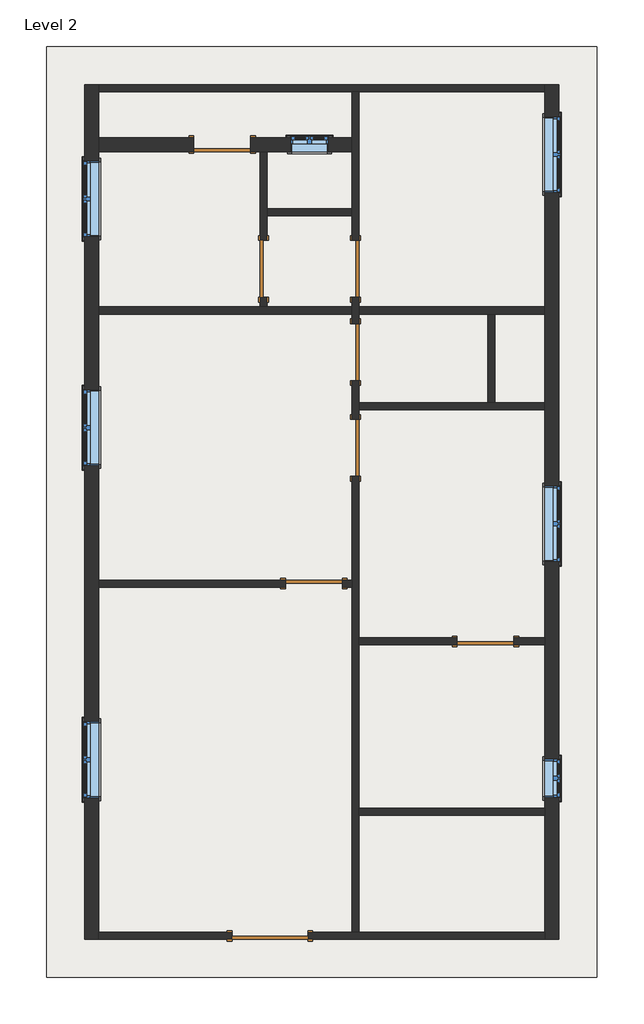
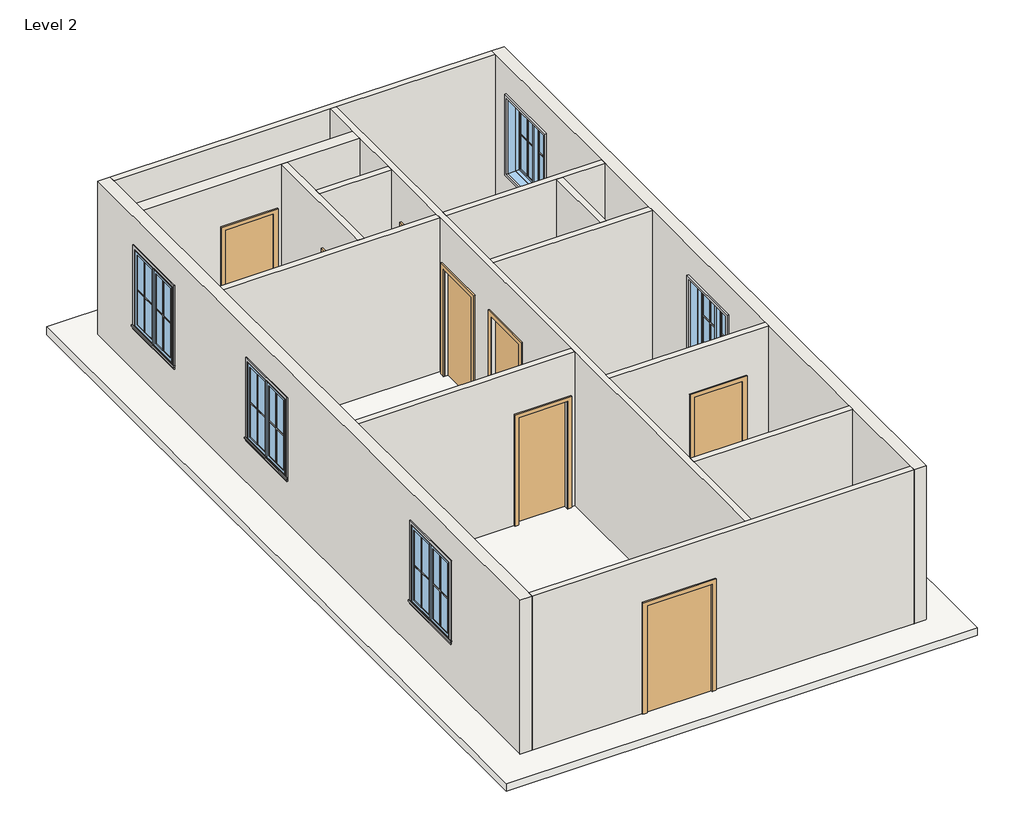
# One storey, incomplete: 28 proxies, 15 walls, 8 doors, 7 windows, 1 slab.
"""IFC4 building model written with IfcOpenShell, lengths in millimetres."""

from ifc_helpers import new_model, si_unit, frame, origin, place, context, project, spatial, polyline, outline, extrude, faceted_brep, transform, mapped, element, save
from components import muntin_pattern_2x2_muntin_pattern_2x2_6dad3731, muntin_pattern_2x2_muntin_pattern_2x2_a30a3345, muntin_pattern_2x2_muntin_pattern_2x2_53152e2c, muntin_pattern_2x2_muntin_pattern_2x2_e8f3e573, trim_window_exterior_flat_with_sill_92b9b949, trim_window_exterior_flat_with_sill_a665a915, trim_window_interior_flat_picture_frame_3bb882cf, trim_window_interior_flat_picture_frame_d485c387, door_a90ba1ad, door_e5f9f3c4, door_305aa2a5, door_6ea84ebe, window_c417fced, window_8377141f

model = new_model("IFC4")

# Units and contexts
model_context = context("Model", 3, world=origin())
ifc_project = project(units=[si_unit("LENGTHUNIT", "METRE", prefix="MILLI")], contexts=[model_context])

# Site, building, storey
site = spatial("IfcSite", under=ifc_project)
building = spatial("IfcBuilding", under=site)
storey = spatial("IfcBuildingStorey", under=building, Name="Level 2", Elevation=3048.0)

# Proxies
placement = place(None, origin())
muntin_pattern_2x2_muntin_pattern_2x2_shape = muntin_pattern_2x2_muntin_pattern_2x2_6dad3731(model_context)
element("IfcBuildingElementProxy", 1, Name="Muntin Pattern_2x2 : Muntin Pattern_2x2", ObjectType="Muntin Pattern_2x2 : Muntin Pattern_2x2", at=placement, inside=storey, context=model_context, shape_type="MappedRepresentation", body=[
    mapped(muntin_pattern_2x2_muntin_pattern_2x2_shape, transform((1279.525, 8669.3375, 4032.25), x_axis=(0.0, 1.0, 0.0), y_axis=(-1.0, 0.0, 0.0), z_axis=(0.0, 0.0, 1.0))),
])
element("IfcBuildingElementProxy", 2, Name="Muntin Pattern_2x2 : Muntin Pattern_2x2", ObjectType="Muntin Pattern_2x2 : Muntin Pattern_2x2", at=placement, inside=storey, context=model_context, shape_type="MappedRepresentation", body=[
    mapped(muntin_pattern_2x2_muntin_pattern_2x2_shape, transform((1279.525, 3341.6875, 4032.25), x_axis=(0.0, 1.0, 0.0), y_axis=(-1.0, 0.0, 0.0), z_axis=(0.0, 0.0, 1.0))),
])
element("IfcBuildingElementProxy", 3, Name="Muntin Pattern_2x2 : Muntin Pattern_2x2", ObjectType="Muntin Pattern_2x2 : Muntin Pattern_2x2", at=placement, inside=storey, context=model_context, shape_type="MappedRepresentation", body=[
    mapped(muntin_pattern_2x2_muntin_pattern_2x2_shape, transform((8880.475, 7732.7125, 4032.25), x_axis=(0.0, -1.0, 0.0), y_axis=(1.0, 0.0, 0.0), z_axis=(0.0, 0.0, 1.0))),
])
element("IfcBuildingElementProxy", 4, Name="Muntin Pattern_2x2 : Muntin Pattern_2x2", ObjectType="Muntin Pattern_2x2 : Muntin Pattern_2x2", at=placement, inside=storey, context=model_context, shape_type="MappedRepresentation", body=[
    mapped(muntin_pattern_2x2_muntin_pattern_2x2_shape, transform((8880.475, 13657.2625, 4032.25), x_axis=(0.0, -1.0, 0.0), y_axis=(1.0, 0.0, 0.0), z_axis=(0.0, 0.0, 1.0))),
])
element("IfcBuildingElementProxy", 5, Name="Muntin Pattern_2x2 : Muntin Pattern_2x2", ObjectType="Muntin Pattern_2x2 : Muntin Pattern_2x2", at=placement, inside=storey, context=model_context, shape_type="MappedRepresentation", body=[
    mapped(muntin_pattern_2x2_muntin_pattern_2x2_shape, transform((1279.525, 12339.6375, 4032.25), x_axis=(0.0, 1.0, 0.0), y_axis=(-1.0, 0.0, 0.0), z_axis=(0.0, 0.0, 1.0))),
])
muntin_pattern_2x2_muntin_pattern_2x2_2_shape = muntin_pattern_2x2_muntin_pattern_2x2_a30a3345(model_context)
element("IfcBuildingElementProxy", 6, Name="Muntin Pattern_2x2 : Muntin Pattern_2x2", ObjectType="Muntin Pattern_2x2 : Muntin Pattern_2x2", at=placement, inside=storey, context=model_context, shape_type="MappedRepresentation", body=[
    mapped(muntin_pattern_2x2_muntin_pattern_2x2_2_shape, transform((1279.525, 9275.7625, 4032.25), x_axis=(0.0, -1.0, 0.0), y_axis=(1.0, 0.0, 0.0), z_axis=(0.0, 0.0, 1.0))),
])
element("IfcBuildingElementProxy", 7, Name="Muntin Pattern_2x2 : Muntin Pattern_2x2", ObjectType="Muntin Pattern_2x2 : Muntin Pattern_2x2", at=placement, inside=storey, context=model_context, shape_type="MappedRepresentation", body=[
    mapped(muntin_pattern_2x2_muntin_pattern_2x2_2_shape, transform((1279.525, 3948.1125, 4032.25), x_axis=(0.0, -1.0, 0.0), y_axis=(1.0, 0.0, 0.0), z_axis=(0.0, 0.0, 1.0))),
])
element("IfcBuildingElementProxy", 8, Name="Muntin Pattern_2x2 : Muntin Pattern_2x2", ObjectType="Muntin Pattern_2x2 : Muntin Pattern_2x2", at=placement, inside=storey, context=model_context, shape_type="MappedRepresentation", body=[
    mapped(muntin_pattern_2x2_muntin_pattern_2x2_2_shape, transform((8880.475, 7126.2875, 4032.25), x_axis=(0.0, 1.0, 0.0), y_axis=(-1.0, 0.0, 0.0), z_axis=(0.0, 0.0, 1.0))),
])
element("IfcBuildingElementProxy", 9, Name="Muntin Pattern_2x2 : Muntin Pattern_2x2", ObjectType="Muntin Pattern_2x2 : Muntin Pattern_2x2", at=placement, inside=storey, context=model_context, shape_type="MappedRepresentation", body=[
    mapped(muntin_pattern_2x2_muntin_pattern_2x2_2_shape, transform((8880.475, 13050.8375, 4032.25), x_axis=(0.0, 1.0, 0.0), y_axis=(-1.0, 0.0, 0.0), z_axis=(0.0, 0.0, 1.0))),
])
element("IfcBuildingElementProxy", 10, Name="Muntin Pattern_2x2 : Muntin Pattern_2x2", ObjectType="Muntin Pattern_2x2 : Muntin Pattern_2x2", at=placement, inside=storey, context=model_context, shape_type="MappedRepresentation", body=[
    mapped(muntin_pattern_2x2_muntin_pattern_2x2_2_shape, transform((1279.525, 12946.0625, 4032.25), x_axis=(0.0, -1.0, 0.0), y_axis=(1.0, 0.0, 0.0), z_axis=(0.0, 0.0, 1.0))),
])
muntin_pattern_2x2_muntin_pattern_2x2_3_shape = muntin_pattern_2x2_muntin_pattern_2x2_53152e2c(model_context)
element("IfcBuildingElementProxy", 11, Name="Muntin Pattern_2x2 : Muntin Pattern_2x2", ObjectType="Muntin Pattern_2x2 : Muntin Pattern_2x2", at=placement, inside=storey, context=model_context, shape_type="MappedRepresentation", body=[
    mapped(muntin_pattern_2x2_muntin_pattern_2x2_3_shape, transform((4732.3375, 13617.575, 4032.25), x_axis=(1.0, 0.0, 0.0), y_axis=(0.0, 1.0, 0.0), z_axis=(0.0, 0.0, 1.0))),
])
element("IfcBuildingElementProxy", 12, Name="Muntin Pattern_2x2 : Muntin Pattern_2x2", ObjectType="Muntin Pattern_2x2 : Muntin Pattern_2x2", at=placement, inside=storey, context=model_context, shape_type="MappedRepresentation", body=[
    mapped(muntin_pattern_2x2_muntin_pattern_2x2_3_shape, transform((8880.475, 3497.2625, 4032.25), x_axis=(0.0, -1.0, 0.0), y_axis=(1.0, 0.0, 0.0), z_axis=(0.0, 0.0, 1.0))),
])
muntin_pattern_2x2_muntin_pattern_2x2_4_shape = muntin_pattern_2x2_muntin_pattern_2x2_e8f3e573(model_context)
element("IfcBuildingElementProxy", 13, Name="Muntin Pattern_2x2 : Muntin Pattern_2x2", ObjectType="Muntin Pattern_2x2 : Muntin Pattern_2x2", at=placement, inside=storey, context=model_context, shape_type="MappedRepresentation", body=[
    mapped(muntin_pattern_2x2_muntin_pattern_2x2_4_shape, transform((5033.9625, 13617.575, 4032.25), x_axis=(-1.0, 0.0, 0.0), y_axis=(0.0, -1.0, 0.0), z_axis=(0.0, 0.0, 1.0))),
])
element("IfcBuildingElementProxy", 14, Name="Muntin Pattern_2x2 : Muntin Pattern_2x2", ObjectType="Muntin Pattern_2x2 : Muntin Pattern_2x2", at=placement, inside=storey, context=model_context, shape_type="MappedRepresentation", body=[
    mapped(muntin_pattern_2x2_muntin_pattern_2x2_4_shape, transform((8880.475, 3195.6375, 4032.25), x_axis=(0.0, 1.0, 0.0), y_axis=(-1.0, 0.0, 0.0), z_axis=(0.0, 0.0, 1.0))),
])
trim_window_exterior_flat_with_sill_shape = trim_window_exterior_flat_with_sill_92b9b949(model_context)
element("IfcBuildingElementProxy", 15, Name="Trim-Window-Exterior-Flat : with Sill", ObjectType="Trim-Window-Exterior-Flat : with Sill", at=placement, inside=storey, context=model_context, shape_type="MappedRepresentation", body=[
    mapped(trim_window_exterior_flat_with_sill_shape, transform((1270.0, 8972.55, 5486.4), x_axis=(0.0, -1.0, 0.0), y_axis=(0.0, 0.0, 1.0), z_axis=(-1.0, 0.0, 0.0))),
])
element("IfcBuildingElementProxy", 16, Name="Trim-Window-Exterior-Flat : with Sill", ObjectType="Trim-Window-Exterior-Flat : with Sill", at=placement, inside=storey, context=model_context, shape_type="MappedRepresentation", body=[
    mapped(trim_window_exterior_flat_with_sill_shape, transform((1270.0, 3644.9, 5486.4), x_axis=(0.0, -1.0, 0.0), y_axis=(0.0, 0.0, 1.0), z_axis=(-1.0, 0.0, 0.0))),
])
element("IfcBuildingElementProxy", 17, Name="Trim-Window-Exterior-Flat : with Sill", ObjectType="Trim-Window-Exterior-Flat : with Sill", at=placement, inside=storey, context=model_context, shape_type="MappedRepresentation", body=[
    mapped(trim_window_exterior_flat_with_sill_shape, transform((8890.0, 7429.5, 5486.4), x_axis=(0.0, 1.0, 0.0), y_axis=(0.0, 0.0, 1.0), z_axis=(1.0, 0.0, 0.0))),
])
element("IfcBuildingElementProxy", 18, Name="Trim-Window-Exterior-Flat : with Sill", ObjectType="Trim-Window-Exterior-Flat : with Sill", at=placement, inside=storey, context=model_context, shape_type="MappedRepresentation", body=[
    mapped(trim_window_exterior_flat_with_sill_shape, transform((8890.0, 13354.05, 5486.4), x_axis=(0.0, 1.0, 0.0), y_axis=(0.0, 0.0, 1.0), z_axis=(1.0, 0.0, 0.0))),
])
element("IfcBuildingElementProxy", 19, Name="Trim-Window-Exterior-Flat : with Sill", ObjectType="Trim-Window-Exterior-Flat : with Sill", at=placement, inside=storey, context=model_context, shape_type="MappedRepresentation", body=[
    mapped(trim_window_exterior_flat_with_sill_shape, transform((1270.0, 12642.85, 5486.4), x_axis=(0.0, -1.0, 0.0), y_axis=(0.0, 0.0, 1.0), z_axis=(-1.0, 0.0, 0.0))),
])
trim_window_exterior_flat_with_sill_2_shape = trim_window_exterior_flat_with_sill_a665a915(model_context)
element("IfcBuildingElementProxy", 20, Name="Trim-Window-Exterior-Flat : with Sill", ObjectType="Trim-Window-Exterior-Flat : with Sill", at=placement, inside=storey, context=model_context, shape_type="MappedRepresentation", body=[
    mapped(trim_window_exterior_flat_with_sill_2_shape, transform((4883.15, 13627.1, 4876.8), x_axis=(-1.0, 0.0, 0.0), y_axis=(0.0, 0.0, 1.0), z_axis=(0.0, 1.0, 0.0))),
])
element("IfcBuildingElementProxy", 21, Name="Trim-Window-Exterior-Flat : with Sill", ObjectType="Trim-Window-Exterior-Flat : with Sill", at=placement, inside=storey, context=model_context, shape_type="MappedRepresentation", body=[
    mapped(trim_window_exterior_flat_with_sill_2_shape, transform((8890.0, 3346.45, 4876.8), x_axis=(0.0, 1.0, 0.0), y_axis=(0.0, 0.0, 1.0), z_axis=(1.0, 0.0, 0.0))),
])
trim_window_interior_flat_picture_frame_shape = trim_window_interior_flat_picture_frame_3bb882cf(model_context)
element("IfcBuildingElementProxy", 22, Name="Trim-Window-Interior-Flat : Picture Frame", ObjectType="Trim-Window-Interior-Flat : Picture Frame", at=placement, inside=storey, context=model_context, shape_type="MappedRepresentation", body=[
    mapped(trim_window_interior_flat_picture_frame_shape, transform((1498.6, 8972.55, 5486.4), x_axis=(0.0, 1.0, 0.0), y_axis=(0.0, 0.0, 1.0), z_axis=(1.0, 0.0, 0.0))),
])
element("IfcBuildingElementProxy", 23, Name="Trim-Window-Interior-Flat : Picture Frame", ObjectType="Trim-Window-Interior-Flat : Picture Frame", at=placement, inside=storey, context=model_context, shape_type="MappedRepresentation", body=[
    mapped(trim_window_interior_flat_picture_frame_shape, transform((1498.6, 3644.9, 5486.4), x_axis=(0.0, 1.0, 0.0), y_axis=(0.0, 0.0, 1.0), z_axis=(1.0, 0.0, 0.0))),
])
element("IfcBuildingElementProxy", 24, Name="Trim-Window-Interior-Flat : Picture Frame", ObjectType="Trim-Window-Interior-Flat : Picture Frame", at=placement, inside=storey, context=model_context, shape_type="MappedRepresentation", body=[
    mapped(trim_window_interior_flat_picture_frame_shape, transform((8661.4, 7429.5, 5486.4), x_axis=(0.0, -1.0, 0.0), y_axis=(0.0, 0.0, 1.0), z_axis=(-1.0, 0.0, 0.0))),
])
element("IfcBuildingElementProxy", 25, Name="Trim-Window-Interior-Flat : Picture Frame", ObjectType="Trim-Window-Interior-Flat : Picture Frame", at=placement, inside=storey, context=model_context, shape_type="MappedRepresentation", body=[
    mapped(trim_window_interior_flat_picture_frame_shape, transform((8661.4, 13354.05, 5486.4), x_axis=(0.0, -1.0, 0.0), y_axis=(0.0, 0.0, 1.0), z_axis=(-1.0, 0.0, 0.0))),
])
element("IfcBuildingElementProxy", 26, Name="Trim-Window-Interior-Flat : Picture Frame", ObjectType="Trim-Window-Interior-Flat : Picture Frame", at=placement, inside=storey, context=model_context, shape_type="MappedRepresentation", body=[
    mapped(trim_window_interior_flat_picture_frame_shape, transform((1498.6, 12642.85, 5486.4), x_axis=(0.0, 1.0, 0.0), y_axis=(0.0, 0.0, 1.0), z_axis=(1.0, 0.0, 0.0))),
])
trim_window_interior_flat_picture_frame_2_shape = trim_window_interior_flat_picture_frame_d485c387(model_context)
element("IfcBuildingElementProxy", 27, Name="Trim-Window-Interior-Flat : Picture Frame", ObjectType="Trim-Window-Interior-Flat : Picture Frame", at=placement, inside=storey, context=model_context, shape_type="MappedRepresentation", body=[
    mapped(trim_window_interior_flat_picture_frame_2_shape, transform((4883.15, 13398.5, 4876.8), x_axis=(1.0, 0.0, 0.0), y_axis=(0.0, 0.0, 1.0), z_axis=(0.0, -1.0, 0.0))),
])
element("IfcBuildingElementProxy", 28, Name="Trim-Window-Interior-Flat : Picture Frame", ObjectType="Trim-Window-Interior-Flat : Picture Frame", at=placement, inside=storey, context=model_context, shape_type="MappedRepresentation", body=[
    mapped(trim_window_interior_flat_picture_frame_2_shape, transform((8661.4, 3346.45, 4876.8), x_axis=(0.0, -1.0, 0.0), y_axis=(0.0, 0.0, 1.0), z_axis=(-1.0, 0.0, 0.0))),
])

# Doors
door_shape = door_a90ba1ad(model_context)
element("IfcDoor", 29, ObjectType="Single-Flush : 36\" x 84\"", at=placement, inside=storey, context=model_context, shape_type="MappedRepresentation", body=[
    mapped(door_shape, transform((3479.8, 13512.8, 3048.0), x_axis=(1.0, 0.0, 0.0), y_axis=(0.0, 1.0, 0.0), z_axis=(0.0, 0.0, 1.0))),
])
door_2_shape = door_e5f9f3c4(model_context)
element("IfcDoor", 30, ObjectType="Single-Flush : 36\" x 84\"", at=placement, inside=storey, context=model_context, shape_type="MappedRepresentation", body=[
    mapped(door_2_shape, transform((5619.75, 11518.9, 3048.0), x_axis=(0.0, -1.0, 0.0), y_axis=(1.0, 0.0, 0.0), z_axis=(0.0, 0.0, 1.0))),
])
element("IfcDoor", 31, ObjectType="Single-Flush : 36\" x 84\"", at=placement, inside=storey, context=model_context, shape_type="MappedRepresentation", body=[
    mapped(door_2_shape, transform((4953.0, 6470.65, 3048.0), x_axis=(1.0, 0.0, 0.0), y_axis=(0.0, 1.0, 0.0), z_axis=(0.0, 0.0, 1.0))),
])
element("IfcDoor", 32, ObjectType="Single-Flush : 36\" x 84\"", at=placement, inside=storey, context=model_context, shape_type="MappedRepresentation", body=[
    mapped(door_2_shape, transform((7708.9, 5543.55, 3048.0), x_axis=(-1.0, 0.0, 0.0), y_axis=(0.0, -1.0, 0.0), z_axis=(0.0, 0.0, 1.0))),
])
door_3_shape = door_305aa2a5(model_context)
element("IfcDoor", 33, ObjectType="Single-Flush : 36\" x 84\"", at=placement, inside=storey, context=model_context, shape_type="MappedRepresentation", body=[
    mapped(door_3_shape, transform((4146.55, 11518.9, 3048.0), x_axis=(0.0, -1.0, 0.0), y_axis=(1.0, 0.0, 0.0), z_axis=(0.0, 0.0, 1.0))),
])
element("IfcDoor", 34, ObjectType="Single-Flush : 36\" x 84\"", at=placement, inside=storey, context=model_context, shape_type="MappedRepresentation", body=[
    mapped(door_3_shape, transform((5619.75, 10185.4, 3048.0), x_axis=(0.0, 1.0, 0.0), y_axis=(-1.0, 0.0, 0.0), z_axis=(0.0, 0.0, 1.0))),
])
element("IfcDoor", 35, ObjectType="Single-Flush : 36\" x 84\"", at=placement, inside=storey, context=model_context, shape_type="MappedRepresentation", body=[
    mapped(door_3_shape, transform((5619.75, 8648.7, 3048.0), x_axis=(0.0, 1.0, 0.0), y_axis=(-1.0, 0.0, 0.0), z_axis=(0.0, 0.0, 1.0))),
])
door_4_shape = door_6ea84ebe(model_context)
element("IfcDoor", 36, ObjectType="Single-Flush : 48\" x 84\"", at=placement, inside=storey, context=model_context, shape_type="MappedRepresentation", body=[
    mapped(door_4_shape, transform((4248.15, 819.15, 3048.0), x_axis=(-1.0, 0.0, 0.0), y_axis=(0.0, -1.0, 0.0), z_axis=(0.0, 0.0, 1.0))),
])

# Slab
element("IfcSlab", 37, ObjectType="Generic - 12\"", at=placement, inside=storey, context=model_context, shape_type="SweptSolid", body=[
    extrude(outline(polyline([(9499.6, 15087.6), (9499.6, 152.4), (660.4, 152.4), (660.4, 15087.6), (9499.6, 15087.6)])), frame((0.0, 0.0, 2895.6), z_axis=(0.0, 0.0, 1.0), x_axis=(1.0, 0.0, 0.0)), (0.0, 0.0, 1.0), 152.4),
])

# Walls
element("IfcWall", 38, ObjectType="Generic - 5\"", at=placement, inside=storey, context=model_context, shape_type="Brep", body=[
    faceted_brep([(1498.6, 14363.7, 3048.0), (5562.6, 14363.7, 3048.0), (5676.9, 14363.7, 3048.0), (8661.4, 14363.7, 3048.0), (8661.4, 14363.7, 6096.0), (5676.9, 14363.7, 6096.0), (5562.6, 14363.7, 6096.0), (1498.6, 14363.7, 6096.0), (1498.6, 14478.0, 3048.0), (1498.6, 14478.0, 6096.0), (8661.4, 14478.0, 6096.0), (8661.4, 14478.0, 3048.0)], [[[0, 1, 2, 3, 4, 5, 6, 7]], [[8, 9, 10, 11]], [[3, 2, 1, 0, 8, 11]], [[7, 6, 5, 4, 10, 9]], [[4, 3, 11, 10]], [[0, 7, 9, 8]]]),
])
element("IfcWall", 39, ObjectType="Generic - 5\"", at=placement, inside=storey, context=model_context, shape_type="Brep", body=[
    faceted_brep([(1498.6, 762.0, 3048.0), (3638.55, 762.0, 3048.0), (3638.55, 762.0, 5181.6), (4857.75, 762.0, 5181.6), (4857.75, 762.0, 3048.0), (8661.4, 762.0, 3048.0), (8661.4, 762.0, 6096.0), (1498.6, 762.0, 6096.0), (3638.55, 876.3, 5181.6), (3638.55, 876.3, 3048.0), (1498.6, 876.3, 3048.0), (1498.6, 876.3, 6096.0), (5562.6, 876.3, 6096.0), (5676.9, 876.3, 6096.0), (8661.4, 876.3, 6096.0), (8661.4, 876.3, 3048.0), (5676.9, 876.3, 3048.0), (5562.6, 876.3, 3048.0), (4857.75, 876.3, 3048.0), (4857.75, 876.3, 5181.6)], [[[0, 1, 2, 3, 4, 5, 6, 7]], [[8, 9, 10, 11, 12, 13, 14, 15, 16, 17, 18, 19]], [[10, 9, 1, 0]], [[18, 17, 16, 15, 5, 4]], [[7, 6, 14, 13, 12, 11]], [[6, 5, 15, 14]], [[0, 7, 11, 10]], [[2, 1, 9, 8]], [[3, 2, 8, 19]], [[4, 3, 19, 18]]]),
])
element("IfcWall", 40, ObjectType="Generic - 5\"", at=placement, inside=storey, context=model_context, shape_type="Brep", body=[
    faceted_brep([(5562.6, 9728.2, 3048.0), (5562.6, 9105.9, 3048.0), (5562.6, 9105.9, 5181.6), (5562.6, 8191.5, 5181.6), (5562.6, 8191.5, 3048.0), (5562.6, 6527.8, 3048.0), (5562.6, 6413.5, 3048.0), (5562.6, 876.3, 3048.0), (5562.6, 876.3, 6096.0), (5562.6, 6413.5, 6096.0), (5562.6, 6527.8, 6096.0), (5562.6, 10795.0, 6096.0), (5562.6, 10909.3, 6096.0), (5562.6, 12369.8, 6096.0), (5562.6, 12484.1, 6096.0), (5562.6, 13398.5, 6096.0), (5562.6, 13627.1, 6096.0), (5562.6, 14363.7, 6096.0), (5562.6, 14363.7, 3048.0), (5562.6, 13627.1, 3048.0), (5562.6, 13398.5, 3048.0), (5562.6, 12484.1, 3048.0), (5562.6, 12369.8, 3048.0), (5562.6, 11976.1, 3048.0), (5562.6, 11976.1, 5181.6), (5562.6, 11061.7, 5181.6), (5562.6, 11061.7, 3048.0), (5562.6, 10909.3, 3048.0), (5562.6, 10795.0, 3048.0), (5562.6, 10642.6, 3048.0), (5562.6, 10642.6, 5181.6), (5562.6, 9728.2, 5181.6), (5676.9, 9105.9, 5181.6), (5676.9, 9105.9, 3048.0), (5676.9, 9258.3, 3048.0), (5676.9, 9372.6, 3048.0), (5676.9, 9728.2, 3048.0), (5676.9, 9728.2, 5181.6), (5676.9, 10642.6, 5181.6), (5676.9, 10642.6, 3048.0), (5676.9, 10795.0, 3048.0), (5676.9, 10909.3, 3048.0), (5676.9, 11061.7, 3048.0), (5676.9, 11061.7, 5181.6), (5676.9, 11976.1, 5181.6), (5676.9, 11976.1, 3048.0), (5676.9, 14363.7, 3048.0), (5676.9, 14363.7, 6096.0), (5676.9, 10909.3, 6096.0), (5676.9, 10795.0, 6096.0), (5676.9, 9372.6, 6096.0), (5676.9, 9258.3, 6096.0), (5676.9, 5600.7, 6096.0), (5676.9, 5486.4, 6096.0), (5676.9, 2870.2, 6096.0), (5676.9, 2755.9, 6096.0), (5676.9, 876.3, 6096.0), (5676.9, 876.3, 3048.0), (5676.9, 2755.9, 3048.0), (5676.9, 2870.2, 3048.0), (5676.9, 5486.4, 3048.0), (5676.9, 5600.7, 3048.0), (5676.9, 8191.5, 3048.0), (5676.9, 8191.5, 5181.6)], [[[0, 1, 2, 3, 4, 5, 6, 7, 8, 9, 10, 11, 12, 13, 14, 15, 16, 17, 18, 19, 20, 21, 22, 23, 24, 25, 26, 27, 28, 29, 30, 31]], [[32, 33, 34, 35, 36, 37, 38, 39, 40, 41, 42, 43, 44, 45, 46, 47, 48, 49, 50, 51, 52, 53, 54, 55, 56, 57, 58, 59, 60, 61, 62, 63]], [[23, 22, 21, 20, 19, 18, 46, 45]], [[42, 41, 40, 39, 29, 28, 27, 26]], [[36, 35, 34, 33, 1, 0]], [[62, 61, 60, 59, 58, 57, 7, 6, 5, 4]], [[17, 16, 15, 14, 13, 12, 11, 10, 9, 8, 56, 55, 54, 53, 52, 51, 50, 49, 48, 47]], [[18, 17, 47, 46]], [[8, 7, 57, 56]], [[43, 42, 26, 25]], [[44, 43, 25, 24]], [[45, 44, 24, 23]], [[30, 29, 39, 38]], [[31, 30, 38, 37]], [[0, 31, 37, 36]], [[2, 1, 33, 32]], [[3, 2, 32, 63]], [[4, 3, 63, 62]]]),
])
element("IfcWall", 41, ObjectType="Generic - 5\"", at=placement, inside=storey, context=model_context, shape_type="SweptSolid", body=[
    extrude(outline(polyline([(3048.0, 5676.9), (3048.0, 7251.7), (5181.6, 7251.7), (5181.6, 8166.1), (3048.0, 8166.1), (3048.0, 8661.4), (6096.0, 8661.4), (6096.0, 5676.9), (3048.0, 5676.9)])), frame((0.0, 5486.4, 0.0), z_axis=(0.0, 1.0, 0.0), x_axis=(0.0, 0.0, 1.0)), (0.0, 0.0, 1.0), 114.3),
])
element("IfcWall", 42, ObjectType="Generic - 5\"", at=placement, inside=storey, context=model_context, shape_type="SweptSolid", body=[
    extrude(outline(polyline([(5181.6, 5410.2), (3048.0, 5410.2), (3048.0, 5562.6), (6096.0, 5562.6), (6096.0, 1498.6), (3048.0, 1498.6), (3048.0, 4495.8), (5181.6, 4495.8), (5181.6, 5410.2)])), frame((0.0, 6413.5, 0.0), z_axis=(0.0, 1.0, 0.0), x_axis=(0.0, 0.0, 1.0)), (0.0, 0.0, 1.0), 114.3),
])
element("IfcWall", 43, ObjectType="Generic - 5\"", at=placement, inside=storey, context=model_context, shape_type="Brep", body=[
    faceted_brep([(1498.6, 10795.0, 3048.0), (5562.6, 10795.0, 3048.0), (5562.6, 10795.0, 6096.0), (1498.6, 10795.0, 6096.0), (1498.6, 10909.3, 3048.0), (1498.6, 10909.3, 6096.0), (4089.4, 10909.3, 6096.0), (4203.7, 10909.3, 6096.0), (5562.6, 10909.3, 6096.0), (5562.6, 10909.3, 3048.0), (4203.7, 10909.3, 3048.0), (4089.4, 10909.3, 3048.0)], [[[0, 1, 2, 3]], [[4, 5, 6, 7, 8, 9, 10, 11]], [[1, 0, 4, 11, 10, 9]], [[3, 2, 8, 7, 6, 5]], [[0, 3, 5, 4]], [[2, 1, 9, 8]]]),
])
element("IfcWall", 44, ObjectType="Generic - 5\"", at=placement, inside=storey, context=model_context, shape_type="Brep", body=[
    faceted_brep([(5676.9, 10795.0, 3048.0), (7747.0010433, 10795.0, 3048.0), (7861.3010433, 10795.0, 3048.0), (8661.4, 10795.0, 3048.0), (8661.4, 10795.0, 6096.0), (7861.3010433, 10795.0, 6096.0), (7747.0010433, 10795.0, 6096.0), (5676.9, 10795.0, 6096.0), (5676.9, 10909.3, 3048.0), (5676.9, 10909.3, 6096.0), (8661.4, 10909.3, 6096.0), (8661.4, 10909.3, 3048.0)], [[[0, 1, 2, 3, 4, 5, 6, 7]], [[8, 9, 10, 11]], [[3, 2, 1, 0, 8, 11]], [[7, 6, 5, 4, 10, 9]], [[4, 3, 11, 10]], [[0, 7, 9, 8]]]),
])
element("IfcWall", 45, ObjectType="Generic - 5\"", at=placement, inside=storey, context=model_context, shape_type="SweptSolid", body=[
    extrude(outline(polyline([(7747.0010433, 9372.6), (7747.0010433, 10795.0), (7861.3010433, 10795.0), (7861.3010433, 9372.6), (7747.0010433, 9372.6)])), frame((0.0, 0.0, 3048.0), z_axis=(0.0, 0.0, 1.0), x_axis=(1.0, 0.0, 0.0)), (0.0, 0.0, 1.0), 3048.0),
])
element("IfcWall", 46, ObjectType="Generic - 5\"", at=placement, inside=storey, context=model_context, shape_type="Brep", body=[
    faceted_brep([(5676.9, 9258.3, 3048.0), (8661.4, 9258.3, 3048.0), (8661.4, 9258.3, 6096.0), (5676.9, 9258.3, 6096.0), (5676.9, 9372.6, 3048.0), (5676.9, 9372.6, 6096.0), (7747.0010433, 9372.6, 6096.0), (7861.3010433, 9372.6, 6096.0), (8661.4, 9372.6, 6096.0), (8661.4, 9372.6, 3048.0), (7861.3010433, 9372.6, 3048.0), (7747.0010433, 9372.6, 3048.0)], [[[0, 1, 2, 3]], [[4, 5, 6, 7, 8, 9, 10, 11]], [[1, 0, 4, 11, 10, 9]], [[3, 2, 8, 7, 6, 5]], [[2, 1, 9, 8]], [[0, 3, 5, 4]]]),
])
element("IfcWall", 47, ObjectType="Generic - 5\"", at=placement, inside=storey, context=model_context, shape_type="SweptSolid", body=[
    extrude(outline(polyline([(8661.4, 2755.9), (5676.9, 2755.9), (5676.9, 2870.2), (8661.4, 2870.2), (8661.4, 2755.9)])), frame((0.0, 0.0, 3048.0), z_axis=(0.0, 0.0, 1.0), x_axis=(1.0, 0.0, 0.0)), (0.0, 0.0, 1.0), 3048.0),
])
element("IfcWall", 48, ObjectType="Generic - 5\"", at=placement, inside=storey, context=model_context, shape_type="Brep", body=[
    faceted_brep([(4203.7, 10909.3, 3048.0), (4203.7, 11061.7, 3048.0), (4203.7, 11061.7, 5181.6), (4203.7, 11976.1, 5181.6), (4203.7, 11976.1, 3048.0), (4203.7, 12369.8, 3048.0), (4203.7, 12484.1, 3048.0), (4203.7, 13398.5, 3048.0), (4203.7, 13398.5, 6096.0), (4203.7, 12484.1, 6096.0), (4203.7, 12369.8, 6096.0), (4203.7, 10909.3, 6096.0), (4089.4, 11061.7, 5181.6), (4089.4, 11061.7, 3048.0), (4089.4, 10909.3, 3048.0), (4089.4, 10909.3, 6096.0), (4089.4, 13398.5, 6096.0), (4089.4, 13398.5, 3048.0), (4089.4, 11976.1, 3048.0), (4089.4, 11976.1, 5181.6)], [[[0, 1, 2, 3, 4, 5, 6, 7, 8, 9, 10, 11]], [[12, 13, 14, 15, 16, 17, 18, 19]], [[18, 17, 7, 6, 5, 4]], [[14, 13, 1, 0]], [[11, 10, 9, 8, 16, 15]], [[0, 11, 15, 14]], [[8, 7, 17, 16]], [[2, 1, 13, 12]], [[3, 2, 12, 19]], [[4, 3, 19, 18]]]),
])
element("IfcWall", 49, ObjectType="Generic - 5\"", at=placement, inside=storey, context=model_context, shape_type="SweptSolid", body=[
    extrude(outline(polyline([(5562.6, 12369.8), (4203.7, 12369.8), (4203.7, 12484.1), (5562.6, 12484.1), (5562.6, 12369.8)])), frame((0.0, 0.0, 3048.0), z_axis=(0.0, 0.0, 1.0), x_axis=(1.0, 0.0, 0.0)), (0.0, 0.0, 1.0), 3048.0),
])
element("IfcWall", 50, ObjectType="Generic - 8\"", at=placement, inside=storey, context=model_context, shape_type="Brep", body=[
    faceted_brep([(8661.4, 14478.0, 3048.0), (8661.4, 14363.7, 3048.0), (8661.4, 10909.3, 3048.0), (8661.4, 10795.0, 3048.0), (8661.4, 9372.6, 3048.0), (8661.4, 9258.3, 3048.0), (8661.4, 5600.7, 3048.0), (8661.4, 5486.4, 3048.0), (8661.4, 2870.2, 3048.0), (8661.4, 2755.9, 3048.0), (8661.4, 876.3, 3048.0), (8661.4, 762.0, 3048.0), (8661.4, 762.0, 6096.0), (8661.4, 876.3, 6096.0), (8661.4, 2755.9, 6096.0), (8661.4, 2870.2, 6096.0), (8661.4, 5486.4, 6096.0), (8661.4, 5600.7, 6096.0), (8661.4, 9258.3, 6096.0), (8661.4, 9372.6, 6096.0), (8661.4, 10795.0, 6096.0), (8661.4, 10909.3, 6096.0), (8661.4, 14363.7, 6096.0), (8661.4, 14478.0, 6096.0), (8661.4, 6819.9, 5486.4), (8661.4, 6819.9, 3962.4), (8661.4, 8039.1, 3962.4), (8661.4, 8039.1, 5486.4), (8661.4, 12744.45, 5486.4), (8661.4, 12744.45, 3962.4), (8661.4, 13963.65, 3962.4), (8661.4, 13963.65, 5486.4), (8661.4, 3041.65, 4876.8), (8661.4, 3041.65, 3962.4), (8661.4, 3651.25, 3962.4), (8661.4, 3651.25, 4876.8), (8890.0, 14478.0, 3048.0), (8890.0, 14478.0, 6096.0), (8890.0, 762.0, 6096.0), (8890.0, 762.0, 3048.0), (8890.0, 6819.9, 5486.4), (8890.0, 8039.1, 5486.4), (8890.0, 8039.1, 3962.4), (8890.0, 6819.9, 3962.4), (8890.0, 12744.45, 5486.4), (8890.0, 13963.65, 5486.4), (8890.0, 13963.65, 3962.4), (8890.0, 12744.45, 3962.4), (8890.0, 3041.65, 4876.8), (8890.0, 3651.25, 4876.8), (8890.0, 3651.25, 3962.4), (8890.0, 3041.65, 3962.4)], [[[0, 1, 2, 3, 4, 5, 6, 7, 8, 9, 10, 11, 12, 13, 14, 15, 16, 17, 18, 19, 20, 21, 22, 23], [24, 25, 26, 27], [28, 29, 30, 31], [32, 33, 34, 35]], [[36, 37, 38, 39], [40, 41, 42, 43], [44, 45, 46, 47], [48, 49, 50, 51]], [[11, 10, 9, 8, 7, 6, 5, 4, 3, 2, 1, 0, 36, 39]], [[23, 22, 21, 20, 19, 18, 17, 16, 15, 14, 13, 12, 38, 37]], [[0, 23, 37, 36]], [[12, 11, 39, 38]], [[25, 24, 40, 43]], [[26, 25, 43, 42]], [[27, 26, 42, 41]], [[24, 27, 41, 40]], [[29, 28, 44, 47]], [[30, 29, 47, 46]], [[31, 30, 46, 45]], [[28, 31, 45, 44]], [[33, 32, 48, 51]], [[34, 33, 51, 50]], [[35, 34, 50, 49]], [[32, 35, 49, 48]]]),
])
element("IfcWall", 51, ObjectType="Generic - 8\"", at=placement, inside=storey, context=model_context, shape_type="Brep", body=[
    faceted_brep([(1270.0, 14478.0, 3048.0), (1270.0, 762.0, 3048.0), (1270.0, 762.0, 6096.0), (1270.0, 14478.0, 6096.0), (1270.0, 9582.15, 5486.4), (1270.0, 8362.95, 5486.4), (1270.0, 8362.95, 3962.4), (1270.0, 9582.15, 3962.4), (1270.0, 4254.5, 5486.4), (1270.0, 3035.3, 5486.4), (1270.0, 3035.3, 3962.4), (1270.0, 4254.5, 3962.4), (1270.0, 13252.45, 5486.4), (1270.0, 12033.25, 5486.4), (1270.0, 12033.25, 3962.4), (1270.0, 13252.45, 3962.4), (1498.6, 14478.0, 3048.0), (1498.6, 14478.0, 6096.0), (1498.6, 14363.7, 6096.0), (1498.6, 13627.1, 6096.0), (1498.6, 13398.5, 6096.0), (1498.6, 10909.3, 6096.0), (1498.6, 10795.0, 6096.0), (1498.6, 6527.8, 6096.0), (1498.6, 6413.5, 6096.0), (1498.6, 876.3, 6096.0), (1498.6, 762.0, 6096.0), (1498.6, 762.0, 3048.0), (1498.6, 876.3, 3048.0), (1498.6, 6413.5, 3048.0), (1498.6, 6527.8, 3048.0), (1498.6, 10795.0, 3048.0), (1498.6, 10909.3, 3048.0), (1498.6, 13398.5, 3048.0), (1498.6, 13627.1, 3048.0), (1498.6, 14363.7, 3048.0), (1498.6, 9582.15, 5486.4), (1498.6, 9582.15, 3962.4), (1498.6, 8362.95, 3962.4), (1498.6, 8362.95, 5486.4), (1498.6, 4254.5, 5486.4), (1498.6, 4254.5, 3962.4), (1498.6, 3035.3, 3962.4), (1498.6, 3035.3, 5486.4), (1498.6, 13252.45, 5486.4), (1498.6, 13252.45, 3962.4), (1498.6, 12033.25, 3962.4), (1498.6, 12033.25, 5486.4)], [[[0, 1, 2, 3], [4, 5, 6, 7], [8, 9, 10, 11], [12, 13, 14, 15]], [[16, 17, 18, 19, 20, 21, 22, 23, 24, 25, 26, 27, 28, 29, 30, 31, 32, 33, 34, 35], [36, 37, 38, 39], [40, 41, 42, 43], [44, 45, 46, 47]], [[1, 0, 16, 35, 34, 33, 32, 31, 30, 29, 28, 27]], [[3, 2, 26, 25, 24, 23, 22, 21, 20, 19, 18, 17]], [[0, 3, 17, 16]], [[2, 1, 27, 26]], [[37, 36, 4, 7]], [[38, 37, 7, 6]], [[39, 38, 6, 5]], [[36, 39, 5, 4]], [[41, 40, 8, 11]], [[42, 41, 11, 10]], [[43, 42, 10, 9]], [[40, 43, 9, 8]], [[45, 44, 12, 15]], [[46, 45, 15, 14]], [[47, 46, 14, 13]], [[44, 47, 13, 12]]]),
])
element("IfcWall", 52, ObjectType="Generic - 8\"", at=placement, inside=storey, context=model_context, shape_type="Brep", body=[
    faceted_brep([(3937.0, 13398.5, 5181.6), (3937.0, 13398.5, 3048.0), (4089.4, 13398.5, 3048.0), (4203.7, 13398.5, 3048.0), (5562.6, 13398.5, 3048.0), (5562.6, 13398.5, 6096.0), (4203.7, 13398.5, 6096.0), (4089.4, 13398.5, 6096.0), (1498.6, 13398.5, 6096.0), (1498.6, 13398.5, 3048.0), (3022.6, 13398.5, 3048.0), (3022.6, 13398.5, 5181.6), (5187.95, 13398.5, 4876.8), (5187.95, 13398.5, 3962.4), (4578.35, 13398.5, 3962.4), (4578.35, 13398.5, 4876.8), (5562.6, 13627.1, 3048.0), (3937.0, 13627.1, 3048.0), (3937.0, 13627.1, 5181.6), (3022.6, 13627.1, 5181.6), (3022.6, 13627.1, 3048.0), (1498.6, 13627.1, 3048.0), (1498.6, 13627.1, 6096.0), (5562.6, 13627.1, 6096.0), (5187.95, 13627.1, 4876.8), (4578.35, 13627.1, 4876.8), (4578.35, 13627.1, 3962.4), (5187.95, 13627.1, 3962.4)], [[[0, 1, 2, 3, 4, 5, 6, 7, 8, 9, 10, 11], [12, 13, 14, 15]], [[16, 17, 18, 19, 20, 21, 22, 23], [24, 25, 26, 27]], [[10, 9, 21, 20]], [[4, 3, 2, 1, 17, 16]], [[8, 7, 6, 5, 23, 22]], [[9, 8, 22, 21]], [[5, 4, 16, 23]], [[18, 17, 1, 0]], [[19, 18, 0, 11]], [[20, 19, 11, 10]], [[13, 12, 24, 27]], [[14, 13, 27, 26]], [[15, 14, 26, 25]], [[12, 15, 25, 24]]]),
])

# Windows
window_shape = window_c417fced(model_context)
element("IfcWindow", 53, ObjectType="Window-Casement-Double : 24\" x 36\"", at=placement, inside=storey, context=model_context, shape_type="MappedRepresentation", body=[
    mapped(window_shape, transform((4883.15, 13512.8, 3048.0), x_axis=(1.0, 0.0, 0.0), y_axis=(0.0, 1.0, 0.0), z_axis=(0.0, 0.0, 1.0))),
])
element("IfcWindow", 54, ObjectType="Window-Casement-Double : 24\" x 36\"", at=placement, inside=storey, context=model_context, shape_type="MappedRepresentation", body=[
    mapped(window_shape, transform((8775.7, 3346.45, 3048.0), x_axis=(0.0, -1.0, 0.0), y_axis=(1.0, 0.0, 0.0), z_axis=(0.0, 0.0, 1.0))),
])
window_2_shape = window_8377141f(model_context)
element("IfcWindow", 55, ObjectType="Window-Casement-Double : 48\" x 60\"", at=placement, inside=storey, context=model_context, shape_type="MappedRepresentation", body=[
    mapped(window_2_shape, transform((1384.3, 8972.55, 3048.0), x_axis=(0.0, 1.0, 0.0), y_axis=(-1.0, 0.0, 0.0), z_axis=(0.0, 0.0, 1.0))),
])
element("IfcWindow", 56, ObjectType="Window-Casement-Double : 48\" x 60\"", at=placement, inside=storey, context=model_context, shape_type="MappedRepresentation", body=[
    mapped(window_2_shape, transform((1384.3, 3644.9, 3048.0), x_axis=(0.0, 1.0, 0.0), y_axis=(-1.0, 0.0, 0.0), z_axis=(0.0, 0.0, 1.0))),
])
element("IfcWindow", 57, ObjectType="Window-Casement-Double : 48\" x 60\"", at=placement, inside=storey, context=model_context, shape_type="MappedRepresentation", body=[
    mapped(window_2_shape, transform((8775.7, 7429.5, 3048.0), x_axis=(0.0, -1.0, 0.0), y_axis=(1.0, 0.0, 0.0), z_axis=(0.0, 0.0, 1.0))),
])
element("IfcWindow", 58, ObjectType="Window-Casement-Double : 48\" x 60\"", at=placement, inside=storey, context=model_context, shape_type="MappedRepresentation", body=[
    mapped(window_2_shape, transform((8775.7, 13354.05, 3048.0), x_axis=(0.0, -1.0, 0.0), y_axis=(1.0, 0.0, 0.0), z_axis=(0.0, 0.0, 1.0))),
])
element("IfcWindow", 59, ObjectType="Window-Casement-Double : 48\" x 60\"", at=placement, inside=storey, context=model_context, shape_type="MappedRepresentation", body=[
    mapped(window_2_shape, transform((1384.3, 12642.85, 3048.0), x_axis=(0.0, 1.0, 0.0), y_axis=(-1.0, 0.0, 0.0), z_axis=(0.0, 0.0, 1.0))),
])

save(model, "model.ifc")

# Revit data of these elements
# Type "Muntin Pattern_2x2 : Muntin Pattern_2x2"
#   Width [instance default] = 4' - 0"
#   Thickness = 0' - 0 1/2"
#   Height [instance default] = 4' - 0"
#   Distance = 0' - 0 3/4"
#   Interior Material [instance default] = none
#   Exterior Material [instance default] = none
#   Default Elevation = 0
# Type "Trim-Window-Exterior-Flat : with Sill"
#   Trim Width = 0' - 2 1/4"
#   Trim Thickness_Picture Frame = 0' - 1 1/4"
#   Trim Thickness_with Sill = 0' - 0 3/4"
#   Sill Thickness = 0' - 1 1/4"
#   Opening Width [instance default] = 2' - 0"
#   Opening Height [instance default] = 3' - 0"
#   Default Elevation = 4' - 0"
#   Sill = yes
#   Picture Frame = no
#   Trim Material [instance default] = none
# Type "Trim-Window-Interior-Flat : Picture Frame"
#   Trim Thickness_Picture Frame = 0' - 1 1/4"
#   Trim Width = 0' - 2 1/4"
#   Trim Thickness_with Sill = 0' - 0 3/4"
#   Sill Thickness = 0' - 1 1/4"
#   Opening Width [instance default] = 2' - 0"
#   Opening Height [instance default] = 3' - 0"
#   Default Elevation = 4' - 0"
#   Sill = no
#   Picture Frame = yes
#   Trim Material [instance default] = none
# Type "Single-Flush : 36\" x 84\""
#   Type Mark = "1"
#   Construction Type Id = "MDOOR"
#   Assembly Code = "C1020"
#   Analytic Construction = "Metal"
#   Thickness = 0' - 2"
#   Heat Transfer Coefficient (U) = 0.651978 BTU/(h·ft²·°F)
#   Height = 7' - 0"
#   Trim Projection Ext = 0' - 1"
#   Trim Projection Int = 0' - 1"
#   Trim Width = 0' - 3"
#   Width = 3' - 0"
#   Define Thermal Properties by = 1
#   Define Thermal Properties by = 1
#   Door Material = Door - Panel
#   Frame Material = Door - Frame
#   Visual Light Transmittance = 0
#   Solar Heat Gain Coefficient = 0
#   Function = (empty or 0)
#   Wall Closure = (empty or 0)
# Type "Single-Flush : 48\" x 84\""
#   Type Mark = "5"
#   Construction Type Id = "MDOOR"
#   Assembly Code = "C1020"
#   Analytic Construction = "Metal"
#   Thickness = 0' - 2"
#   Heat Transfer Coefficient (U) = 0.651978 BTU/(h·ft²·°F)
#   Height = 7' - 0"
#   Trim Projection Ext = 0' - 1"
#   Trim Projection Int = 0' - 1"
#   Trim Width = 0' - 3"
#   Width = 4' - 0"
#   Define Thermal Properties by = 1
#   Define Thermal Properties by = 1
#   Door Material = Door - Panel
#   Frame Material = Door - Frame
#   Visual Light Transmittance = 0
#   Solar Heat Gain Coefficient = 0
#   Function = (empty or 0)
#   Wall Closure = (empty or 0)
# Type "Generic - 12\""
#   Assembly Code = "B1010"
#   Function = 0
#   Layers, outside or top first: 0' - 6" no material (function 1)
# Type "Generic - 5\""
#   Assembly Code = "B2010"
#   Layers, outside or top first: 0' - 4 1/2" no material (function 1)
# Type "Generic - 8\""
#   Assembly Code = "B2010"
#   Layers, outside or top first: 0' - 9" no material (function 1)
# Type "Window-Casement-Double : 24\" x 36\""
#   Type Mark = "14"
#   Fire Rating = "0.5h"
#   Assembly Code = "B2020100"
#   Analytic Construction = "Double glazing - domestic"
#   Frame Extension [instance default] = 0' - 0 1/4"
#   Window Inset [instance default] = 0' - 0"
#   Wall Thickness [instance default] = 0' - 6"
#   Interior Wall Closure [instance default] = 0' - 2 1/4"
#   Half Width = 1' - 0"
#   Visual Light Transmittance = 0.81
#   Thermal Resistance (R) = 1.8146 (h·ft²·°F)/BTU
#   Solar Heat Gain Coefficient = 0.76
#   Rough Width = 2' - 0 1/2"
#   Rough Height = 3' - 0 1/2"
#   Height = 3' - 0"
#   Heat Transfer Coefficient (U) = 0.5511 BTU/(h·ft²·°F)
#   Exterior Wall Closure [instance default] = 0' - 1 1/4"
#   Extension Jamb [instance default] = 0' - 2 1/4"
#   Default Sill Height = 3' - 0"
#   Width = 2' - 0"
#   Define Thermal Properties by = 0
#   Muntin Visibility = yes
#   Interior Trim Visibility [instance default] = yes
#   Exterior Trim Visibility [instance default] = yes
#   Extension Jamb Visibility [instance default] = yes
#   Interior Trim Material = Wood - Stained
#   Muntin Pattern = Muntin Pattern_2x2 : Muntin Pattern_2x2
#   Interior Trim = Trim-Window-Interior-Flat : Picture Frame
#   Interior Frame Material = Wood - Stained
#   Glass Panel Material = Glass
#   Exterior Trim Material = Clad - White
#   Exterior Trim = Trim-Window-Exterior-Flat : with Sill
#   Exterior Frame Material = Clad - White
#   Wall Closure = (empty or 0)
# Type "Window-Casement-Double : 48\" x 60\""
#   Type Mark = "17"
#   Fire Rating = "0.5h"
#   Assembly Code = "B2020100"
#   Analytic Construction = "Double glazing - domestic"
#   Frame Extension [instance default] = 0' - 0 1/4"
#   Window Inset [instance default] = 0' - 0"
#   Wall Thickness [instance default] = 0' - 6"
#   Interior Wall Closure [instance default] = 0' - 2 1/4"
#   Half Width = 2' - 0"
#   Visual Light Transmittance = 0.81
#   Thermal Resistance (R) = 1.8146 (h·ft²·°F)/BTU
#   Solar Heat Gain Coefficient = 0.76
#   Rough Width = 4' - 0 1/2"
#   Rough Height = 5' - 0 1/2"
#   Height = 5' - 0"
#   Heat Transfer Coefficient (U) = 0.5511 BTU/(h·ft²·°F)
#   Exterior Wall Closure [instance default] = 0' - 1 1/4"
#   Extension Jamb [instance default] = 0' - 2 1/4"
#   Default Sill Height = 3' - 0"
#   Width = 4' - 0"
#   Define Thermal Properties by = 0
#   Muntin Visibility = yes
#   Interior Trim Visibility [instance default] = yes
#   Exterior Trim Visibility [instance default] = yes
#   Extension Jamb Visibility [instance default] = yes
#   Interior Trim Material = Wood - Stained
#   Muntin Pattern = Muntin Pattern_2x2 : Muntin Pattern_2x2
#   Interior Trim = Trim-Window-Interior-Flat : Picture Frame
#   Interior Frame Material = Wood - Stained
#   Glass Panel Material = Glass
#   Exterior Trim Material = Clad - White
#   Exterior Trim = Trim-Window-Exterior-Flat : with Sill
#   Exterior Frame Material = Clad - White
#   Wall Closure = (empty or 0)
# Elements 1, 2, 3, 4, 5, 6, 7, 8, 9, 10 (IfcBuildingElementProxy, "Muntin Pattern_2x2 : Muntin Pattern_2x2")
#   Width = 1' - 6 5/8"
#   Height = 4' - 6 1/2"
#   Interior Material = Wood - Stained
#   Exterior Material = Clad - White
#   Phase Created = New Construction
#   Materials on its faces: "Clad - White", "Wood - Stained"
# Elements 11, 12, 13, 14 (IfcBuildingElementProxy, "Muntin Pattern_2x2 : Muntin Pattern_2x2")
#   Width = 0' - 6 5/8"
#   Height = 2' - 6 1/2"
#   Interior Material = Wood - Stained
#   Exterior Material = Clad - White
#   Phase Created = New Construction
#   Materials on its faces: "Clad - White", "Wood - Stained"
# Elements 15, 16, 17, 18, 19 (IfcBuildingElementProxy, "Trim-Window-Exterior-Flat : with Sill")
#   Opening Width = 4' - 0"
#   Opening Height = 5' - 0"
#   Trim Material = Clad - White
#   Phase Created = New Construction
#   Materials on its faces: "Clad - White"
# Elements 20, 21 (IfcBuildingElementProxy, "Trim-Window-Exterior-Flat : with Sill")
#   Opening Width = 2' - 0"
#   Opening Height = 3' - 0"
#   Trim Material = Clad - White
#   Phase Created = New Construction
#   Materials on its faces: "Clad - White"
# Elements 22, 23, 24, 25, 26 (IfcBuildingElementProxy, "Trim-Window-Interior-Flat : Picture Frame")
#   Opening Width = 4' - 0"
#   Opening Height = 5' - 0"
#   Trim Material = Wood - Stained
#   Phase Created = New Construction
#   Materials on its faces: "Wood - Stained"
# Elements 27, 28 (IfcBuildingElementProxy, "Trim-Window-Interior-Flat : Picture Frame")
#   Opening Width = 2' - 0"
#   Opening Height = 3' - 0"
#   Trim Material = Wood - Stained
#   Phase Created = New Construction
#   Materials on its faces: "Wood - Stained"
# Elements 29, 30, 31, 32, 33, 34, 35 (IfcDoor, "Single-Flush : 36\" x 84\"")
#   Phase Created = New Construction
#   Materials on its faces: "Door - Frame", "Door - Panel"
# Element 36 (IfcDoor, "Single-Flush : 48\" x 84\"")
#   Phase Created = New Construction
#   Materials on its faces: "Door - Frame", "Door - Panel"
# Element 37 (IfcSlab, "Generic - 12\"")
#   Height Offset From Level = 0' - 0"
#   Phase Created = New Construction
#   Materials on its faces: "Clad - White", "Default Floor"
# Elements 38, 39 (IfcWall, "Generic - 5\"")
#   Top Offset = 0' - 0"
#   Base Offset = 0' - 0"
#   wall height = 10' - 0"
#   Phase Created = New Construction
#   Base Constraint = Level 2
#   Top Constraint = Level 3
#   Materials on its faces: "Default Wall", "Parking Stripe"
# Elements 40, 41, 42, 43, 44, 45, 46, 47, 48, 49 (IfcWall, "Generic - 5\"")
#   Top Offset = 0' - 0"
#   Base Offset = 0' - 0"
#   wall height = 10' - 0"
#   Phase Created = New Construction
#   Base Constraint = Level 2
#   Top Constraint = Level 3
#   Materials on its faces: "Default Wall"
# Element 50 (IfcWall, "Generic - 8\"")
#   Top Offset = 0' - 0"
#   Base Offset = 0' - 0"
#   Unconnected Height = 10' - 0"
#   wall height = 10' - 0"
#   Phase Created = New Construction
#   Base Constraint = Level 2
#   Materials on its faces: "Default Wall", "Parking Stripe", "Plywood, Sheathing"
# Element 51 (IfcWall, "Generic - 8\"")
#   Top Offset = 0' - 0"
#   Base Offset = 0' - 0"
#   Unconnected Height = 10' - 0"
#   wall height = 10' - 0"
#   Phase Created = New Construction
#   Base Constraint = Level 2
#   Materials on its faces: "Default Wall", "Parking Stripe"
# Element 52 (IfcWall, "Generic - 8\"")
#   Top Offset = 0' - 0"
#   Base Offset = 0' - 0"
#   Unconnected Height = 10' - 0"
#   wall height = 10' - 0"
#   Phase Created = New Construction
#   Base Constraint = Level 2
#   Materials on its faces: "Default Wall"
# Element 53 (IfcWindow, "Window-Casement-Double : 24\" x 36\"")
#   Mark = "20"
#   Window Inset = 0' - 0"
#   Interior Wall Closure = 0' - 2 1/4"
#   Frame Extension = 0' - 0 1/4"
#   Exterior Wall Closure = 0' - 1 1/4"
#   Interior Trim Visibility = yes
#   Exterior Trim Visibility = yes
#   Phase Created = New Construction
#   Materials on its faces: "Wood - Stained", "Glass", "Clad - White"
# Element 54 (IfcWindow, "Window-Casement-Double : 24\" x 36\"")
#   Mark = "21"
#   Window Inset = 0' - 0"
#   Interior Wall Closure = 0' - 2 1/4"
#   Frame Extension = 0' - 0 1/4"
#   Exterior Wall Closure = 0' - 1 1/4"
#   Interior Trim Visibility = yes
#   Exterior Trim Visibility = yes
#   Phase Created = New Construction
#   Materials on its faces: "Wood - Stained", "Glass", "Clad - White"
# Element 55 (IfcWindow, "Window-Casement-Double : 48\" x 60\"")
#   Mark = "15"
#   Window Inset = 0' - 0"
#   Interior Wall Closure = 0' - 2 1/4"
#   Frame Extension = 0' - 0 1/4"
#   Exterior Wall Closure = 0' - 1 1/4"
#   Interior Trim Visibility = yes
#   Exterior Trim Visibility = yes
#   Phase Created = New Construction
#   Materials on its faces: "Wood - Stained", "Glass", "Clad - White"
# Element 56 (IfcWindow, "Window-Casement-Double : 48\" x 60\"")
#   Mark = "16"
#   Window Inset = 0' - 0"
#   Interior Wall Closure = 0' - 2 1/4"
#   Frame Extension = 0' - 0 1/4"
#   Exterior Wall Closure = 0' - 1 1/4"
#   Interior Trim Visibility = yes
#   Exterior Trim Visibility = yes
#   Phase Created = New Construction
#   Materials on its faces: "Wood - Stained", "Glass", "Clad - White"
# Element 57 (IfcWindow, "Window-Casement-Double : 48\" x 60\"")
#   Mark = "17"
#   Window Inset = 0' - 0"
#   Interior Wall Closure = 0' - 2 1/4"
#   Frame Extension = 0' - 0 1/4"
#   Exterior Wall Closure = 0' - 1 1/4"
#   Interior Trim Visibility = yes
#   Exterior Trim Visibility = yes
#   Phase Created = New Construction
#   Materials on its faces: "Wood - Stained", "Glass", "Clad - White"
# Element 58 (IfcWindow, "Window-Casement-Double : 48\" x 60\"")
#   Mark = "18"
#   Window Inset = 0' - 0"
#   Interior Wall Closure = 0' - 2 1/4"
#   Frame Extension = 0' - 0 1/4"
#   Exterior Wall Closure = 0' - 1 1/4"
#   Interior Trim Visibility = yes
#   Exterior Trim Visibility = yes
#   Phase Created = New Construction
#   Materials on its faces: "Wood - Stained", "Glass", "Clad - White"
# Element 59 (IfcWindow, "Window-Casement-Double : 48\" x 60\"")
#   Mark = "19"
#   Window Inset = 0' - 0"
#   Interior Wall Closure = 0' - 2 1/4"
#   Frame Extension = 0' - 0 1/4"
#   Exterior Wall Closure = 0' - 1 1/4"
#   Interior Trim Visibility = yes
#   Exterior Trim Visibility = yes
#   Phase Created = New Construction
#   Materials on its faces: "Wood - Stained", "Glass", "Clad - White"
# Materials
#   "Door - Panel": class "Wood", colour RGB 210 159 95, transparency 0, Cost = 0
#   "Door - Frame": colour RGB 118 70 51, transparency 0, Cost = 0
#   "Wood - Stained": class "Wood", colour RGB 224 178 126, transparency 0, Cost = 0
#   "Glass": class "Glass", colour RGB 0 128 192, transparency 0.75, Description = "Soda Lime Glass", Cost = 0
#   "Clad - White": class "Wood", colour RGB 242 242 238, transparency 0, Cost = 0
#   "Default Floor": colour RGB 128 128 128, transparency 0, Cost = 0
#   "Default Wall": colour RGB 128 128 128, transparency 0, Cost = 0
#   "Parking Stripe": class "Paint", colour RGB 250 250 91, transparency 0, Cost = 0
#   "Plywood, Sheathing": class "Wood", colour RGB 212 179 113, transparency 0, Description = "Plywood, sheathing grade", Cost = 0
